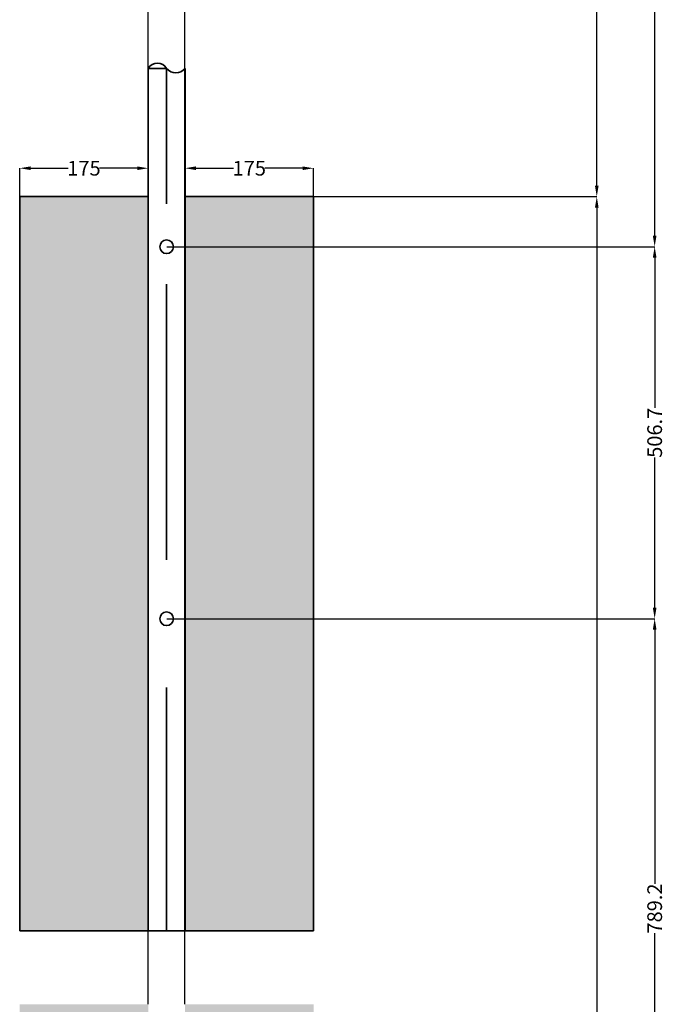
# Model space of a CAD drawing. Units: inches. Extents: x -129 to 2013, y -3652 to 814.
# Tile 4 of 5: x 805 to 1683, y -1868 to -527. Entities that reach past the tile are written whole.
import ezdxf

# ---------------------------------------------------------------- set-up
doc = ezdxf.new("R2010")
doc.units = ezdxf.units.IN
doc.header["$MEASUREMENT"] = 0
for name, color, linetype, lineweight in [('A-ANNO-DIMS', 2, 'Continuous', 18), ('A-DETL', 7, 'Continuous', 35), ('A-DETL-PATT', 8, 'Continuous', 13), ('E-GRND', 1, 'Continuous', 35)]:
    doc.layers.add(name, color=color, linetype=linetype, lineweight=lineweight)
doc.styles.get("Standard").update_dxf_attribs({"font": 'arial.ttf'})
doc.dimstyles.get("Standard").update_dxf_attribs({"dimtxt": 20, "dimasz": 15, "dimexe": 0.18, "dimexo": 0.0625, "dimgap": 0.09, "dimtad": 0, "dimdec": 0, "dimzin": 0, "dimdsep": 46, "dimtxsty": 'Standard', "dimcen": 0.09, "dimadec": 0, "dimazin": 0, "dimtfac": 1, "dimtdec": 0, "dimtofl": 0, "dimtmove": 0, "dimatfit": 3, "dimfxl": 1, "dimtolj": 1, "dimtzin": 0, "dimarcsym": 0})

# ---------------------------------------------------------------- blocks, each defined once
blk = doc.blocks.new('*D2')
at = {"layer": 'A-ANNO-DIMS', "color": 0, "lineweight": -2, "transparency": 16777216}
for p, q in [((1330.4, 482.4), (1591, 482.4)), ((1590.8, 467.4), (1590.8, -113.7)), ((1590.8, -752.6), (1590.8, -171.6)), ((1205.4, -767.6), (1591, -767.6))]:
    blk.add_line(p, q, dxfattribs=at)
at = {"layer": 'A-ANNO-DIMS', "color": 0, "transparency": 16777216}
for points in [[(1588.3, 467.4), (1593.3, 467.4), (1590.8, 482.4)], [(1588.3, -752.6), (1593.3, -752.6), (1590.8, -767.6)]]:
    blk.add_solid(points, dxfattribs=at)
at = {"layer": 'Defpoints', "color": 0, "transparency": 16777216}
for p in [(1330.3, 482.4), (1205.3, -767.6), (1590.8, -767.6)]:
    blk.add_point(p, dxfattribs=at)
at = {"layer": 'A-ANNO-DIMS', "color": 0, "transparency": 16777216, "insert": (1590.8, -142.6), "char_height": 20, "attachment_point": 5, "rotation": 90}
blk.add_mtext('\\A1;1250', dxfattribs=at)
blk = doc.blocks.new('*D3')
at = {"layer": 'A-ANNO-DIMS', "color": 0, "lineweight": -2, "transparency": 16777216}
for p, q in [((1205.4, -767.6), (1591, -767.6)), ((1590.8, -782.6), (1590.8, -1987.5)), ((1590.8, -3252.6), (1590.8, -2047.7)), ((1205.4, -3267.6), (1591, -3267.6))]:
    blk.add_line(p, q, dxfattribs=at)
at = {"layer": 'A-ANNO-DIMS', "color": 0, "transparency": 16777216}
for points in [[(1588.3, -782.6), (1593.3, -782.6), (1590.8, -767.6)], [(1588.3, -3252.6), (1593.3, -3252.6), (1590.8, -3267.6)]]:
    blk.add_solid(points, dxfattribs=at)
at = {"layer": 'Defpoints', "color": 0, "transparency": 16777216}
for p in [(1205.3, -767.6), (1205.3, -3267.6), (1590.8, -3267.6)]:
    blk.add_point(p, dxfattribs=at)
at = {"layer": 'A-ANNO-DIMS', "color": 0, "transparency": 16777216, "insert": (1590.8, -2017.6), "char_height": 20, "attachment_point": 5, "rotation": 90}
blk.add_mtext('\\A1;2500', dxfattribs=at)
blk = doc.blocks.new('*D9')
at = {"layer": 'A-ANNO-DIMS', "color": 0, "lineweight": -2, "transparency": 16777216}
for p, q in [((805.3, -767.6), (805.3, -728.8)), ((820.3, -729), (871.5, -729)), ((965.3, -729), (914.1, -729)), ((980.3, -767.6), (980.3, -728.8))]:
    blk.add_line(p, q, dxfattribs=at)
at = {"layer": 'A-ANNO-DIMS', "color": 0, "transparency": 16777216}
for points in [[(820.3, -726.5), (820.3, -731.5), (805.3, -729)], [(965.3, -726.5), (965.3, -731.5), (980.3, -729)]]:
    blk.add_solid(points, dxfattribs=at)
at = {"layer": 'Defpoints', "color": 0, "transparency": 16777216}
for p in [(805.3, -729), (805.3, -767.6), (980.3, -767.6)]:
    blk.add_point(p, dxfattribs=at)
at = {"layer": 'A-ANNO-DIMS', "color": 0, "transparency": 16777216, "insert": (892.8, -729), "char_height": 20, "attachment_point": 5}
blk.add_mtext('\\A1;175', dxfattribs=at)
blk = doc.blocks.new('*D10')
at = {"layer": 'A-ANNO-DIMS', "color": 0, "lineweight": -2, "transparency": 16777216}
for p, q in [((1030.3, -767.6), (1030.3, -728.8)), ((1045.3, -729), (1096.5, -729)), ((1190.3, -729), (1139.1, -729)), ((1205.3, -767.6), (1205.3, -728.8))]:
    blk.add_line(p, q, dxfattribs=at)
at = {"layer": 'A-ANNO-DIMS', "color": 0, "transparency": 16777216}
for points in [[(1045.3, -726.5), (1045.3, -731.5), (1030.3, -729)], [(1190.3, -726.5), (1190.3, -731.5), (1205.3, -729)]]:
    blk.add_solid(points, dxfattribs=at)
at = {"layer": 'Defpoints', "color": 0, "transparency": 16777216}
for p in [(1205.3, -729), (1030.3, -767.6), (1205.3, -767.6)]:
    blk.add_point(p, dxfattribs=at)
at = {"layer": 'A-ANNO-DIMS', "color": 0, "transparency": 16777216, "insert": (1117.8, -729), "char_height": 20, "attachment_point": 5}
blk.add_mtext('\\A1;175', dxfattribs=at)
blk = doc.blocks.new('*D26')
at = {"layer": 'A-ANNO-DIMS', "color": 0, "lineweight": -2, "transparency": 16777216}
for p, q in [((980.3, -1867.6), (980.3, 801.3)), ((995.3, 801.1), (1015.3, 801.1)), ((1030.3, -1867.6), (1030.3, 801.3)), ((1030.3, 801.1), (1045.3, 801.1))]:
    blk.add_line(p, q, dxfattribs=at)
at = {"layer": 'A-ANNO-DIMS', "color": 0, "transparency": 16777216}
for points in [[(995.3, 803.6), (995.3, 798.6), (980.3, 801.1)], [(1015.3, 803.6), (1015.3, 798.6), (1030.3, 801.1)]]:
    blk.add_solid(points, dxfattribs=at)
at = {"layer": 'Defpoints', "color": 0, "transparency": 16777216}
for p in [(1030.3, 801.1), (980.3, -1867.6), (1030.3, -1867.6)]:
    blk.add_point(p, dxfattribs=at)
at = {"layer": 'A-ANNO-DIMS', "color": 0, "transparency": 16777216, "insert": (1059.7, 801.1), "char_height": 20, "attachment_point": 5}
blk.add_mtext('\\A1;50', dxfattribs=at)
blk = doc.blocks.new('*D29')
at = {"layer": 'A-ANNO-DIMS', "color": 0, "lineweight": -2, "transparency": 16777216}
for p, q in [((1005.4, 64.7), (1669.8, 64.7)), ((1669.6, 49.7), (1669.6, -351.8)), ((1669.6, -821), (1669.6, -419.5)), ((1005.4, -836), (1669.8, -836))]:
    blk.add_line(p, q, dxfattribs=at)
at = {"layer": 'A-ANNO-DIMS', "color": 0, "transparency": 16777216}
for points in [[(1667.1, 49.7), (1672.1, 49.7), (1669.6, 64.7)], [(1667.1, -821), (1672.1, -821), (1669.6, -836)]]:
    blk.add_solid(points, dxfattribs=at)
at = {"layer": 'Defpoints', "color": 0, "transparency": 16777216}
for p in [(1005.3, 64.7), (1005.3, -836), (1669.6, -836)]:
    blk.add_point(p, dxfattribs=at)
at = {"layer": 'A-ANNO-DIMS', "color": 0, "transparency": 16777216, "insert": (1669.6, -385.6), "char_height": 20, "attachment_point": 5, "rotation": 90}
blk.add_mtext('\\A1;900.7', dxfattribs=at)
blk = doc.blocks.new('*D30')
at = {"layer": 'A-ANNO-DIMS', "color": 0, "lineweight": -2, "transparency": 16777216}
for p, q in [((1005.4, -836), (1669.8, -836)), ((1669.6, -851), (1669.6, -1055.5)), ((1669.6, -1327.6), (1669.6, -1123.1)), ((1005.4, -1342.6), (1669.8, -1342.6))]:
    blk.add_line(p, q, dxfattribs=at)
at = {"layer": 'A-ANNO-DIMS', "color": 0, "transparency": 16777216}
for points in [[(1667.1, -851), (1672.1, -851), (1669.6, -836)], [(1667.1, -1327.6), (1672.1, -1327.6), (1669.6, -1342.6)]]:
    blk.add_solid(points, dxfattribs=at)
at = {"layer": 'Defpoints', "color": 0, "transparency": 16777216}
for p in [(1005.3, -836), (1005.3, -1342.6), (1669.6, -1342.6)]:
    blk.add_point(p, dxfattribs=at)
at = {"layer": 'A-ANNO-DIMS', "color": 0, "transparency": 16777216, "insert": (1669.6, -1089.3), "char_height": 20, "attachment_point": 5, "rotation": 90}
blk.add_mtext('\\A1;506.7', dxfattribs=at)
blk = doc.blocks.new('*D31')
at = {"layer": 'A-ANNO-DIMS', "color": 0, "lineweight": -2, "transparency": 16777216}
for p, q in [((1005.4, -1342.6), (1669.8, -1342.6)), ((1669.6, -1357.6), (1669.6, -1703.6)), ((1669.6, -2116.9), (1669.6, -1770.9)), ((1005.4, -2131.9), (1669.8, -2131.9))]:
    blk.add_line(p, q, dxfattribs=at)
at = {"layer": 'A-ANNO-DIMS', "color": 0, "transparency": 16777216}
for points in [[(1667.1, -1357.6), (1672.1, -1357.6), (1669.6, -1342.6)], [(1667.1, -2116.9), (1672.1, -2116.9), (1669.6, -2131.9)]]:
    blk.add_solid(points, dxfattribs=at)
at = {"layer": 'Defpoints', "color": 0, "transparency": 16777216}
for p in [(1005.3, -1342.6), (1005.3, -2131.9), (1669.6, -2131.9)]:
    blk.add_point(p, dxfattribs=at)
at = {"layer": 'A-ANNO-DIMS', "color": 0, "transparency": 16777216, "insert": (1669.6, -1737.2), "char_height": 20, "attachment_point": 5, "rotation": 90}
blk.add_mtext('\\A1;789.2', dxfattribs=at)

msp = doc.modelspace()

# ---------------------------------------------------------------- hatches: boundary and pattern name
at = {"layer": 'A-DETL-PATT'}
h = msp.add_hatch(dxfattribs=at)
h.set_pattern_fill('AR-CONC', color=256, scale=10)
h.paths.add_polyline_path([(1205.3299, -767.6397), (1030.3299, -767.6397), (1030.3299, -1767.6397), (1205.3299, -1767.6397)])
h.paths.add_polyline_path([(980.3299, -767.6397), (805.3299, -767.6397), (805.3299, -1767.6397), (980.3299, -1767.6397)])
h.paths.add_polyline_path([(980.3299, -1867.6397), (805.3299, -1867.6397), (805.3299, -3267.6397), (1205.3299, -3267.6397), (1205.3299, -1867.6397), (1030.3299, -1867.6397), (1030.3299, -2970.3227), (980.3299, -2907.6958)])

# ---------------------------------------------------------------- linework, layer by layer
at = {"layer": 'A-DETL'}
for p, q in [((805.3299, -767.6397), (805.3299, -1767.6397)), ((980.3299, -767.6397), (805.3299, -767.6397)), ((1205.3299, -767.6397), (1030.3299, -767.6397)), ((1205.3299, -767.6397), (1205.3299, -1767.6397)), ((1205.3299, -1767.6397), (805.3299, -1767.6397))]:
    msp.add_line(p, q, dxfattribs=at)
at = {"layer": 'E-GRND'}
for p, q in [((980.3299, -593.0431), (1005.3299, -593.0431)), ((980.3299, -593.0431), (980.3299, -1767.6397)), ((1005.3299, -593.0431), (1005.3299, -777.4389)), ((1030.3299, -593.0431), (1030.3299, -1767.6397)), ((1005.3299, -886.8112), (1005.3299, -1262.3034)), ((1005.3299, -1436.2128), (1005.3299, -1767.6397))]:
    msp.add_line(p, q, dxfattribs=at)
for centre in [(1005.3299, -835.9565), (1005.3299, -1342.6284)]:
    msp.add_circle(centre, 9.277, dxfattribs=at)
for centre, radius, start, end in [((992.8299, -600.0138), 14.3122, 29.1463796, 150.8536204), ((1017.8299, -583.4219), 15.774, 217.5854091, 322.4145909)]:
    msp.add_arc(centre, radius, start, end, dxfattribs=at)

# ---------------------------------------------------------------- dimensions: what is measured, and where the dimension line sits
at = {"layer": 'A-ANNO-DIMS'}
for base, p1, p2, override, picture, middle in [((1030.3299, 801.1186), (980.3299, -1867.6397), (1030.3299, -1867.6397), {"dimdec": 0, "dimlfac": 1, "dimrnd": 0, "dimzin": 0, "dimdsep": 46, "dimlunit": 2}, '*D26', (1059.7105, 801.1186)), ((805.3299, -728.956), (980.3299, -767.6397), (805.3299, -767.6397), {"dimclrd": 0, "dimclre": 0, "dimclrt": 0}, '*D9', (892.8299, -728.956)), ((1205.3299, -728.956), (1030.3299, -767.6397), (1205.3299, -767.6397), {"dimclrd": 0, "dimclre": 0, "dimclrt": 0}, '*D10', (1117.8299, -728.956))]:
    dim = msp.add_linear_dim(base=base, p1=p1, p2=p2, dimstyle='Standard', override=override, dxfattribs=at)
    dim.commit()
    dim.dimension.update_dxf_attribs({"geometry": picture, "text_midpoint": middle})
for base, p1, p2, override, picture, middle in [((1590.798, -767.6397), (1330.3299, 482.3603), (1205.3299, -767.6397), {"dimclrd": 0, "dimclre": 0, "dimclrt": 0}, '*D2', (1590.798, -142.6397)), ((1669.5799, -835.9565), (1005.3299, 64.711), (1005.3299, -835.9565), {"dimdec": 1, "dimlfac": 1, "dimrnd": 0, "dimzin": 0, "dimdsep": 46, "dimlunit": 2}, '*D29', (1669.5799, -385.6228)), ((1590.798, -3267.6397), (1205.3299, -767.6397), (1205.3299, -3267.6397), {"dimclrd": 0, "dimclre": 0, "dimclrt": 0}, '*D3', (1590.798, -2017.6397)), ((1669.5799, -1342.6284), (1005.3299, -835.9565), (1005.3299, -1342.6284), {"dimdec": 1, "dimlfac": 1, "dimrnd": 0, "dimzin": 0, "dimdsep": 46, "dimlunit": 2}, '*D30', (1669.5799, -1089.2924)), ((1669.5799, -2131.8545), (1005.3299, -1342.6284), (1005.3299, -2131.8545), {"dimdec": 1, "dimlfac": 1, "dimrnd": 0, "dimzin": 0, "dimdsep": 46, "dimlunit": 2}, '*D31', (1669.5799, -1737.2414))]:
    dim = msp.add_linear_dim(base=base, p1=p1, p2=p2, angle=90, dimstyle='Standard', override=override, dxfattribs=at)
    dim.commit()
    dim.dimension.update_dxf_attribs({"geometry": picture, "text_midpoint": middle})

doc.saveas('drawing.dxf')
